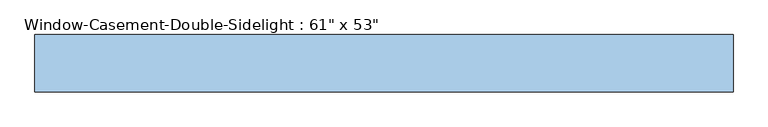
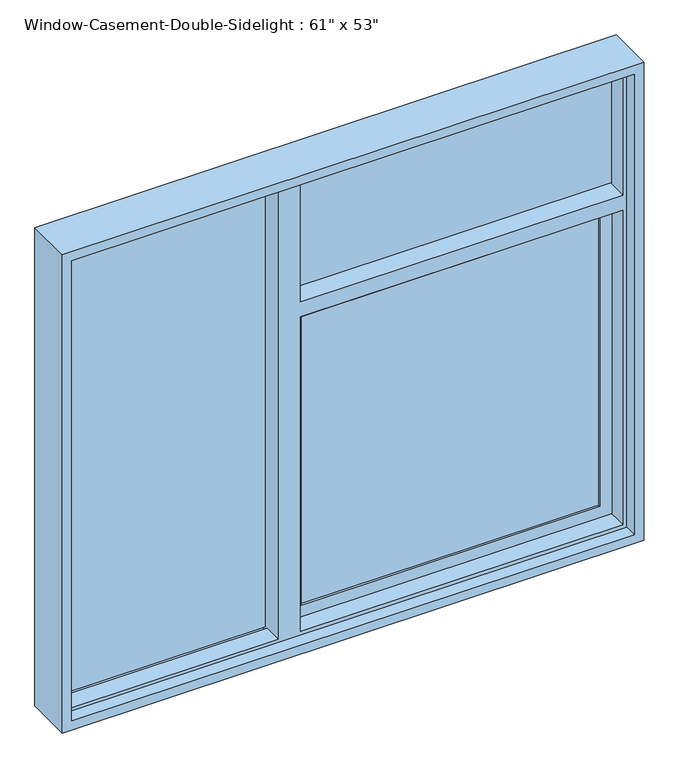
"""IFC4 building model written with IfcOpenShell, lengths in millimetres: window geometry."""

from ifc_helpers import new_model, si_unit, frame, origin, place, context, project, spatial, polyline, outline, extrude, faceted_brep, source, transform, mapped, element, save


def window_5c3f3b46(model_context):
    return source(origin(), model_context, "Body", "SolidModel", [
        extrude(outline(polyline([(707.4296875, 47.625), (-87.6696875, 47.625), (-87.6696875, 60.325), (707.4296875, 60.325), (707.4296875, 47.625)])), frame((0.0, 0.0, 981.6703125), z_axis=(0.0, 0.0, 1.0), x_axis=(1.0, 0.0, 0.0)), (0.0, 0.0, 1.0), 812.2642187),
        extrude(outline(polyline([(707.4296875, 34.925), (707.4296875, 28.575), (-87.6696875, 28.575), (-87.6696875, 34.925), (707.4296875, 34.925)])), frame((0.0, 0.0, 981.6703125), z_axis=(0.0, 0.0, 1.0), x_axis=(1.0, 0.0, 0.0)), (0.0, 0.0, 1.0), 812.2642187),
        extrude(outline(polyline([(-180.34, 47.625), (-180.34, 41.275), (-749.3, 41.275), (-749.3, 47.625), (-180.34, 47.625)])), frame((0.0, 0.0, 949.9203125), z_axis=(0.0, 0.0, 1.0), x_axis=(1.0, 0.0, 0.0)), (0.0, 0.0, 1.0), 1285.2796875),
        extrude(outline(polyline([(-180.34, 34.925), (-180.34, 28.575), (-749.3, 28.575), (-749.3, 34.925), (-180.34, 34.925)])), frame((0.0, 0.0, 949.9203125), z_axis=(0.0, 0.0, 1.0), x_axis=(1.0, 0.0, 0.0)), (0.0, 0.0, 1.0), 1285.2796875),
        extrude(outline(polyline([(749.3, 34.925), (749.3, 28.575), (-129.54, 28.575), (-129.54, 34.925), (749.3, 34.925)])), frame((0.0, 0.0, 1877.6751563), z_axis=(0.0, 0.0, 1.0), x_axis=(1.0, 0.0, 0.0)), (0.0, 0.0, 1.0), 357.5248438),
        extrude(outline(polyline([(749.3, 47.625), (749.3, 41.275), (-129.54, 41.275), (-129.54, 47.625), (749.3, 47.625)])), frame((0.0, 0.0, 1877.6751563), z_axis=(0.0, 0.0, 1.0), x_axis=(1.0, 0.0, 0.0)), (0.0, 0.0, 1.0), 357.5248438),
        faceted_brep([(-749.3, 22.225, 2235.2), (-749.3, 63.5, 2235.2), (749.3, 63.5, 2235.2), (749.3, 22.225, 2235.2), (-129.54, 22.225, 2235.2), (-129.54, 60.325, 2235.2), (-180.34, 60.325, 2235.2), (-180.34, 22.225, 2235.2), (-739.1796875, -28.575, 2225.0796875), (-739.1796875, 22.225, 2225.0796875), (-180.34, 22.225, 2225.0796875), (-180.34, -28.575, 2225.0796875), (739.1796875, 22.225, 2225.0796875), (739.1796875, -28.575, 2225.0796875), (-119.4196875, -28.575, 2225.0796875), (-119.4196875, 22.225, 2225.0796875), (-749.3, -63.5, 2235.2), (-749.3, -28.575, 2235.2), (749.3, -28.575, 2235.2), (749.3, -63.5, 2235.2), (-774.7, 63.5, 2260.6), (-774.7, -63.5, 2260.6), (774.7, -63.5, 2260.6), (774.7, 63.5, 2260.6), (749.3, 63.5, 939.8), (749.3, 22.225, 939.8), (749.3, 22.225, 1835.8048438), (749.3, 60.325, 1835.8048438), (749.3, 60.325, 1877.6751563), (749.3, 22.225, 1877.6751563), (739.1796875, 22.225, 1877.6751563), (739.1796875, -28.575, 1877.6751563), (739.1796875, 22.225, 949.9203125), (739.1796875, -28.575, 949.9203125), (739.1796875, -28.575, 1835.8048438), (739.1796875, 22.225, 1835.8048438), (749.3, -28.575, 939.8), (749.3, -63.5, 939.8), (774.7, -63.5, 914.4), (774.7, 63.5, 914.4), (-749.3, 63.5, 939.8), (-749.3, 22.225, 939.8), (-180.34, 22.225, 939.8), (-180.34, 60.325, 939.8), (-129.54, 60.325, 939.8), (-129.54, 22.225, 939.8), (-119.4196875, 22.225, 949.9203125), (-119.4196875, -28.575, 949.9203125), (-739.1796875, 22.225, 949.9203125), (-739.1796875, -28.575, 949.9203125), (-180.34, -28.575, 949.9203125), (-180.34, 22.225, 949.9203125), (-749.3, -28.575, 939.8), (-749.3, -63.5, 939.8), (-774.7, -63.5, 914.4), (-774.7, 63.5, 914.4), (-119.4196875, 22.225, 1877.6751563), (-129.54, 22.225, 1877.6751563), (-129.54, 22.225, 1835.8048438), (-119.4196875, 22.225, 1835.8048438), (-119.4196875, -28.575, 1877.6751563), (-119.4196875, -28.575, 1835.8048438), (-129.54, 60.325, 1877.6751563), (-129.54, 60.325, 1835.8048438)], [[[0, 1, 2, 3, 4, 5, 6, 7]], [[8, 9, 10, 11]], [[12, 13, 14, 15]], [[16, 17, 18, 19]], [[20, 21, 22, 23]], [[3, 2, 24, 25, 26, 27, 28, 29]], [[13, 12, 30, 31]], [[32, 33, 34, 35]], [[19, 18, 36, 37]], [[23, 22, 38, 39]], [[25, 24, 40, 41, 42, 43, 44, 45]], [[33, 32, 46, 47]], [[48, 49, 50, 51]], [[37, 36, 52, 53]], [[39, 38, 54, 55]], [[1, 0, 41, 40]], [[12, 15, 56, 57, 4, 3, 29, 30]], [[46, 32, 35, 26, 25, 45, 58, 59]], [[41, 0, 7, 10, 9, 48, 51, 42]], [[9, 8, 49, 48]], [[17, 52, 36, 18], [13, 31, 60, 14], [33, 47, 61, 34], [49, 8, 11, 50]], [[17, 16, 53, 52]], [[22, 21, 54, 38], [16, 19, 37, 53]], [[21, 20, 55, 54]], [[20, 23, 39, 55], [2, 1, 40, 24]], [[43, 6, 5, 62, 28, 27, 63, 44]], [[6, 43, 42, 51, 50, 11, 10, 7]], [[15, 14, 60, 56]], [[47, 46, 59, 61]], [[5, 4, 57, 62]], [[45, 44, 63, 58]], [[63, 27, 26, 35, 34, 61, 59, 58]], [[28, 62, 57, 56, 60, 31, 30, 29]]]),
        extrude(outline(polyline([(1835.8048438, 749.3), (1835.8048438, -129.54), (939.8, -129.54), (939.8, 749.3), (1835.8048438, 749.3)]), holes=[polyline([(981.6703125, 707.4296875), (981.6703125, -87.6696875), (1793.9345313, -87.6696875), (1793.9345313, 707.4296875), (981.6703125, 707.4296875)])]), frame((0.0, 22.225, 0.0), z_axis=(0.0, 1.0, 0.0), x_axis=(0.0, 0.0, 1.0)), (0.0, 0.0, 1.0), 31.75),
    ])


if __name__ == "__main__":
    model = new_model("IFC4")
    model_context = context("Model", 3, world=origin())
    ifc_project = project(units=[si_unit("LENGTHUNIT", "METRE", prefix="MILLI")], contexts=[model_context])
    site = spatial("IfcSite", under=ifc_project)
    building = spatial("IfcBuilding", under=site)
    placement = place(None, origin())
    window_shape = window_5c3f3b46(model_context)
    element("IfcWindow", 1, ObjectType="Window-Casement-Double-Sidelight : 61\" x 53\"", at=placement, inside=building, context=model_context, shape_type="MappedRepresentation", body=[
        mapped(window_shape, transform((0.0, 0.0, 0.0), x_axis=(1.0, 0.0, 0.0), y_axis=(0.0, 1.0, 0.0), z_axis=(0.0, 0.0, 1.0))),
    ])
    save(model, "model.ifc")

# Revit data of these elements
# Type "Window-Casement-Double-Sidelight : 61\" x 53\""
#   Type Mark = "55"
#   Fire Rating = "0.5h"
#   Assembly Code = "B2020100"
#   Analytic Construction = "Double glazing - domestic"
#   Window Inset [instance default] = 0' - 0 5/8"
#   Wall Thickness [instance default] = 0' - 6"
#   Visual Light Transmittance = 0.81
#   Transom Height Ratio = 0.3
#   Transom Height = 1' - 3.9"
#   Thermal Resistance (R) = 0.319569 (m²·K)/W
#   Solar Heat Gain Coefficient = 0.76
#   Side Width = 2' - 0.4"
#   Rough Width = 5' - 1 1/2"
#   Rough Height = 4' - 5 1/2"
#   Opening Window Width = 3' - 0.6"
#   Opening Window Height = 3' - 1.1"
#   Heat Transfer Coefficient (U) = 3.12929 W/(m²·K)
#   Height = 4' - 5"
#   Frame Gap 3 [instance default] = 0' - 1 83/128"
#   Frame Gap 2 [instance default] = 0' - 0 5/8"
#   Frame Gap 1 = 0' - 1 51/128"
#   Default Sill Height = 3' - 0"
#   Width = 5' - 1"
#   Frame Material = Metal - Aluminum
#   Glass Panel Material = Glass
#   Wall Closure = (empty or 0)
# Element 1 (IfcWindow, "Window-Casement-Double-Sidelight : 61\" x 53\"")
#   Wall Thickness = 0' - 5"
#   Materials on its faces: "Metal - Aluminum", "Glass"
# Materials
#   "Metal - Aluminum": class "Metal", colour RGB 247 247 247, transparency 0
#   "Glass": class "Glass", colour RGB 0 128 192, transparency 0.9, Description = "Soda Lime Glass", Cost = 0
